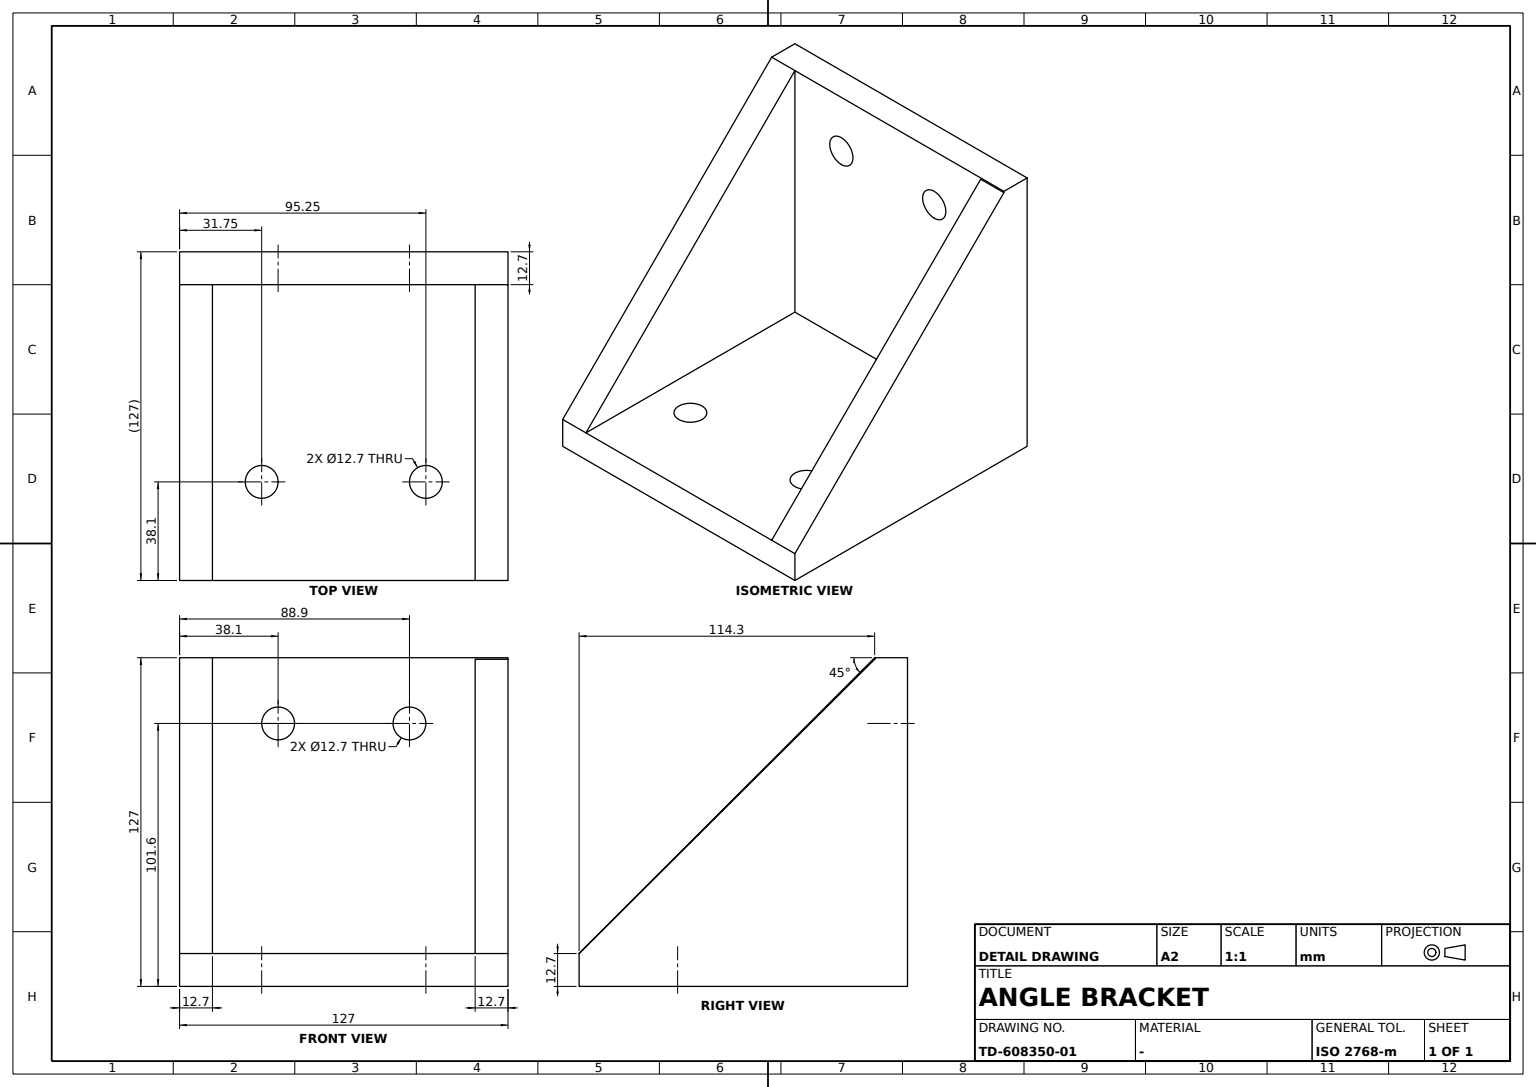
CATIA V5 part; units mm, degrees
sketch "Sketch1" plane through (0, 0, 0) normal (0, 0, 1) x (1, 0, 0)
  line L0 (63.5, 63.5) -> (63.5, -63.5)
  line L1 (63.5, -63.5) -> (-63.5, -63.5)
  line L2 (-63.5, -63.5) -> (-63.5, 63.5)
  line L3 (-63.5, 63.5) -> (63.5, 63.5)
  point P0 (31.75, -25.4)
  circle A0 centre (-31.75, -25.4) radius 6.35
  circle A1 centre (31.75, -25.4) radius 6.35
  dimension "distance L1 L3" = 127
  dimension "distance L0 L2" = 127
  dimension "distance P0 L3" = 88.9
  dimension "radius A0" = 6.35
  constraint vertical L0 y-axis
  constraint vertical L2 y-axis
  constraint horizontal L1 x-axis
  constraint horizontal L3 x-axis
  constraint equidistance L0 L2 origin
  constraint equidistance L1 L3 origin
  constraint symmetry A0 A1 y-axis
extrude "Pad1" add sketch "Sketch1" along normal blind 12.7
sketch "Sketch2" plane through (0, 0, 12.7) normal (0, 0, 1) x (1, 0, 0)
  line L0 (63.5, 63.5) -> (63.5, 50.8)
  line L1 (63.5, 50.8) -> (-63.5, 50.8)
  line L2 (-63.5, 50.8) -> (-63.5, 63.5)
  line L3 (-63.5, 63.5) -> (63.5, 63.5)
  dimension "length L0" = 12.7
  constraint vertical L0 y-axis
  constraint vertical L2 y-axis
  constraint horizontal L1 x-axis
  constraint horizontal L3 x-axis
extrude "Pad2" add sketch "Sketch2" along normal blind 114.3
sketch "Sketch3" plane through (0, 50.8, 0) normal (0, -1, 0) x (1, 0, 0)
  circle A0 centre (-25.4, 101.6) radius 6.35
  point P0 (-25.4, 101.6)
  line L0 (-63.5, 0) -> (63.5, 0) construction
  circle A1 centre (25.4, 101.6) radius 6.35
  dimension "distance P0 L0" = 101.6
  dimension "distance P0 y axis" = 25.4
  constraint symmetry A0 A1 y-axis
extrude "Pocket1" cut sketch "Sketch3" against normal through all
sketch "Sketch4" plane through (63.5, 0, 0) normal (1, 0, 0) x (0, 1, 0)
  line L0 (-63.5, 12.7) -> (50.8, 126.38)
  line L1 (50.8, 126.38) -> (50.8, 12.7)
  line L2 (50.8, 12.7) -> (-63.5, 12.7)
  constraint vertical L1 y-axis
  constraint horizontal L2 x-axis
extrude "Pad3" add sketch "Sketch4" against normal blind 12.7
sketch "Sketch6" plane through (-63.5, 0, 0) normal (-1, 0, 0) x (0, -1, 0)
  line L0 (-50.8, 127) -> (63.5, 12.7)
  line L1 (63.5, 12.7) -> (-50.8, 12.7)
  line L2 (-50.8, 12.7) -> (-50.8, 127)
  constraint horizontal L1 x-axis
  constraint vertical L2 y-axis
extrude "Pad4" add sketch "Sketch6" against normal blind 12.7
sketch "Sketch5" plane through (-63.5, 0, 0) normal (-1, 0, 0) x (0, -1, 0)
